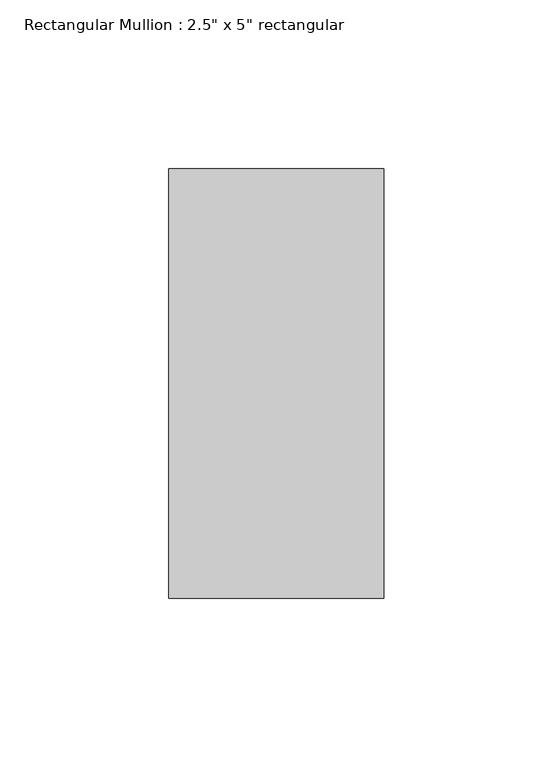
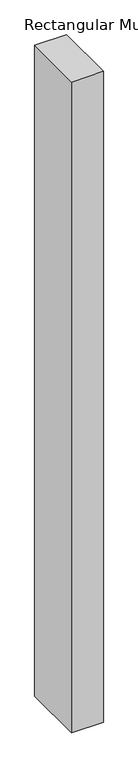
"""IFC4 building model written with IfcOpenShell, lengths in millimetres: member geometry."""

from ifc_helpers import new_model, si_unit, frame, origin, place, context, project, spatial, polyline, outline, extrude, source, transform, mapped, element, save


def member_08a74848(model_context):
    return source(origin(), model_context, "Body", "SweptSolid", [
        extrude(outline(polyline([(31.75, 63.5), (31.75, -63.5), (-31.75, -63.5), (-31.75, 63.5), (31.75, 63.5)])), frame((0.0, 0.0, -1371.5999998), z_axis=(0.0, 0.0, 1.0), x_axis=(1.0, 0.0, 0.0)), (0.0, 0.0, 1.0), 1371.5999998),
    ])


if __name__ == "__main__":
    model = new_model("IFC4")
    model_context = context("Model", 3, world=origin())
    ifc_project = project(units=[si_unit("LENGTHUNIT", "METRE", prefix="MILLI")], contexts=[model_context])
    site = spatial("IfcSite", under=ifc_project)
    building = spatial("IfcBuilding", under=site)
    placement = place(None, origin())
    member_shape = member_08a74848(model_context)
    element("IfcMember", 1, ObjectType="Rectangular Mullion : 2.5\" x 5\" rectangular", at=placement, inside=building, context=model_context, shape_type="MappedRepresentation", body=[
        mapped(member_shape, transform((0.0, 0.0, 0.0), x_axis=(1.0, 0.0, 0.0), y_axis=(0.0, 1.0, 0.0), z_axis=(0.0, 0.0, 1.0))),
    ])
    save(model, "model.ifc")

# Revit data of these elements
# Type "Rectangular Mullion : 2.5\" x 5\" rectangular"
#   built-in parameter 1007304 = 0.416667 (stored number, unit not read)
#   built-in parameter 1007301 = 0.104167 (stored number, unit not read)
#   built-in parameter 1007300 = 0.104167 (stored number, unit not read)
# Element 1 (IfcMember, "Rectangular Mullion : 2.5\" x 5\" rectangular")
#   Materials on its faces: "Aluminum"
# Materials
#   "Aluminum": class "Metal", colour RGB 247 247 247, transparency 0, Description = "Aluminum 6061", Cost = 0
